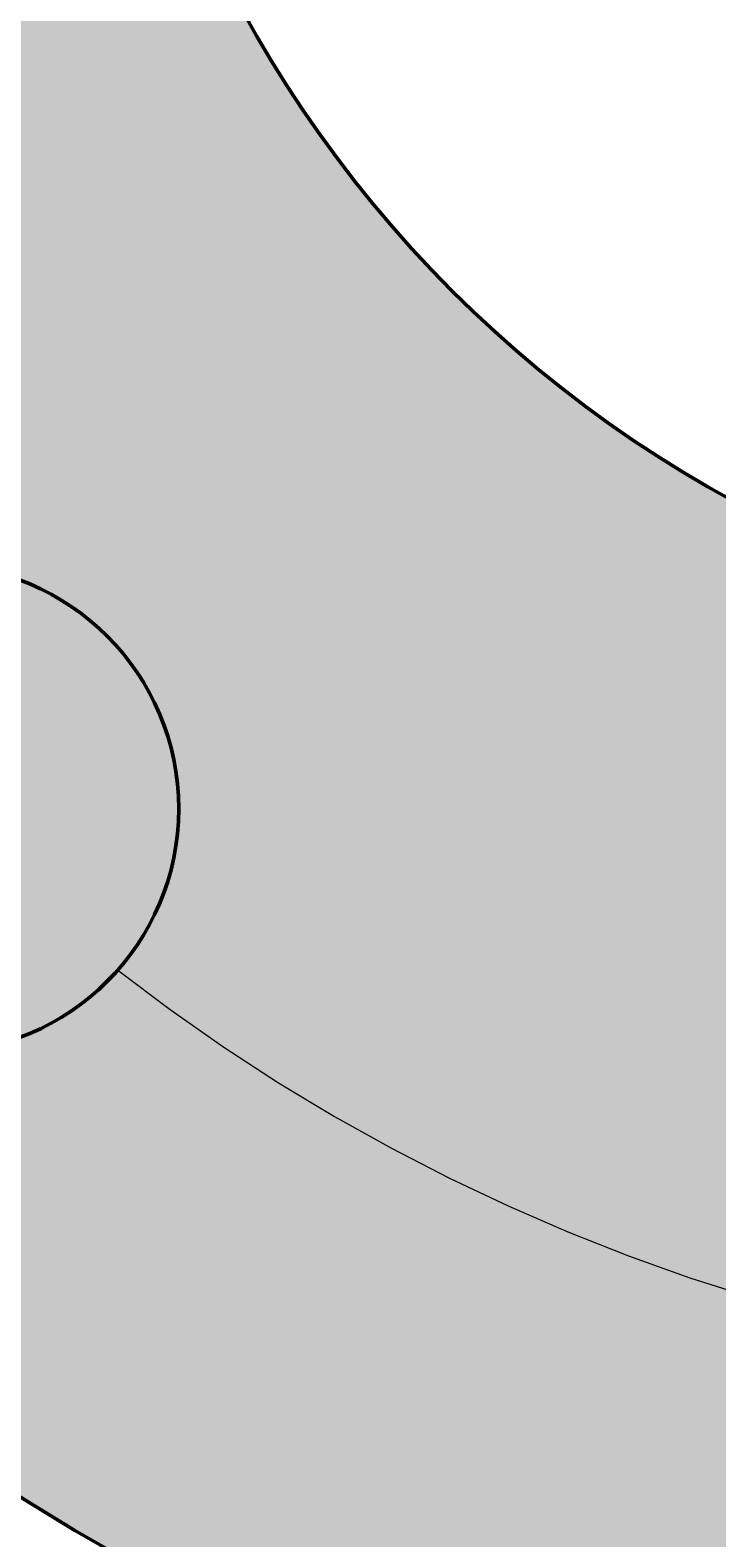
# Model space of a CAD drawing. Units: inches. Extents: x 139261 to 139415, y 52839 to 52963.
# Tile 8 of 20: x 139314 to 139328, y 52857 to 52888. Entities that reach past the tile are written whole.
import ezdxf

# ---------------------------------------------------------------- set-up
doc = ezdxf.new("R2010")
doc.units = ezdxf.units.IN
doc.header["$MEASUREMENT"] = 0
doc.linetypes.add('CENTER', pattern=[50.8, 31.75, -6.35, 6.35, -6.35])
for name, color, linetype, lineweight in [('M-CNTR', 4, 'CENTER', 18), ('M-DIMS', 2, 'Continuous', 25), ('M-HATC', 8, 'Continuous', 18), ('M-OUTL', 7, 'Continuous', 50)]:
    doc.layers.add(name, color=color, linetype=linetype, lineweight=lineweight)
doc.styles.get("Standard").update_dxf_attribs({"font": 'arial.ttf'})
doc.dimstyles.get("Standard").update_dxf_attribs({"dimtxt": 0.18, "dimasz": 0.18, "dimexe": 0.18, "dimexo": 0.0625, "dimgap": 0.09, "dimtad": 0, "dimtih": 1, "dimtoh": 1, "dimdec": 4, "dimzin": 0, "dimdsep": 46, "dimtxsty": 'Standard', "dimcen": 0.09, "dimadec": 0, "dimazin": 0, "dimtfac": 1, "dimtdec": 4, "dimtofl": 0, "dimtmove": 0, "dimatfit": 3, "dimfxl": 1, "dimtolj": 1, "dimtzin": 0, "dimarcsym": 0})

# ---------------------------------------------------------------- blocks, each defined once
blk = doc.blocks.new('*U1')
blk.add_circle((0, 0), 5)
blk = doc.blocks.new('*U2')
at = {"layer": 'M-OUTL', "color": 0, "linetype": 'ByBlock', "lineweight": -2, "transparency": 16777216, "rotation": 135}
blk.add_blockref('*U1', (139312.073, 52871.933), dxfattribs=at)
blk = doc.blocks.new('*D4')
at = {"layer": 'Defpoints', "color": 0, "transparency": 16777216}
for p in [(139373.053, 52923.26), (139307.661, 52877.175)]:
    blk.add_point(p, dxfattribs=at)
at = {"layer": 'M-DIMS', "color": 0, "lineweight": -2, "transparency": 16777216}
for p, q in [((139414.011, 52952.126), (139373.2, 52923.364)), ((139414.191, 52952.126), (139414.011, 52952.126)), ((139340.357, 52900.127), (139340.357, 52900.307)), ((139340.267, 52900.217), (139340.447, 52900.217))]:
    blk.add_line(p, q, dxfattribs=at)
blk.add_arc((139340.357, 52900.217), 40, 34.9168, 52.0771, dxfattribs=at)
at = {"layer": 'M-DIMS', "color": 0, "transparency": 16777216}
blk.add_solid([(139373.183, 52923.388), (139373.217, 52923.339), (139373.053, 52923.26)], dxfattribs=at)
at = {"layer": 'M-DIMS', "color": 0, "transparency": 16777216, "insert": (139414.822, 52952.126), "char_height": 0.18, "attachment_point": 5}
blk.add_mtext('\\A1;∅80.0000', dxfattribs=at)
blk = doc.blocks.new('*D7')
at = {"layer": 'Defpoints', "color": 0, "transparency": 16777216}
for p in [(139316.56, 52874.138), (139307.585, 52869.728)]:
    blk.add_point(p, dxfattribs=at)
at = {"layer": 'M-DIMS', "color": 0, "lineweight": -2, "transparency": 16777216}
for p, q in [((139311.983, 52871.933), (139312.163, 52871.933)), ((139312.073, 52871.843), (139312.073, 52872.023)), ((139282.904, 52857.598), (139307.424, 52869.649)), ((139282.724, 52857.598), (139282.904, 52857.598))]:
    blk.add_line(p, q, dxfattribs=at)
at = {"layer": 'M-DIMS', "color": 0, "transparency": 16777216}
blk.add_solid([(139307.41, 52869.675), (139307.437, 52869.622), (139307.585, 52869.728)], dxfattribs=at)
at = {"layer": 'M-DIMS', "color": 0, "transparency": 16777216, "insert": (139282.093, 52857.598), "char_height": 0.18, "attachment_point": 5}
blk.add_mtext('\\A1;∅10.0000', dxfattribs=at)
blk = doc.blocks.new('*D9')
at = {"layer": 'Defpoints', "color": 0, "transparency": 16777216}
for p in [(139302.054, 52932.357), (139378.659, 52868.078)]:
    blk.add_point(p, dxfattribs=at)
at = {"layer": 'M-DIMS', "color": 0, "lineweight": -2, "transparency": 16777216}
for p, q in [((139278.893, 52951.64), (139279.073, 52951.64)), ((139279.073, 52951.64), (139301.916, 52932.472)), ((139340.357, 52900.127), (139340.357, 52900.307)), ((139340.267, 52900.217), (139340.447, 52900.217))]:
    blk.add_line(p, q, dxfattribs=at)
at = {"layer": 'M-DIMS', "color": 0, "transparency": 16777216}
blk.add_solid([(139301.936, 52932.495), (139301.897, 52932.449), (139302.054, 52932.357)], dxfattribs=at)
at = {"layer": 'M-DIMS', "color": 0, "transparency": 16777216, "insert": (139278.506, 52951.64), "char_height": 0.18, "attachment_point": 5}
blk.add_mtext('\\A1;∅100', dxfattribs=at)
blk = doc.blocks.new('*D10')
at = {"layer": 'Defpoints', "color": 0, "transparency": 16777216}
for p in [(139325.07, 52937.181), (139355.644, 52863.254)]:
    blk.add_point(p, dxfattribs=at)
at = {"layer": 'M-DIMS', "color": 0, "lineweight": -2, "transparency": 16777216}
for p, q in [((139340.357, 52900.127), (139340.357, 52900.307)), ((139340.267, 52900.217), (139340.447, 52900.217)), ((139364.816, 52841.075), (139355.712, 52863.087)), ((139364.996, 52841.075), (139364.816, 52841.075))]:
    blk.add_line(p, q, dxfattribs=at)
at = {"layer": 'M-DIMS', "color": 0, "transparency": 16777216}
blk.add_solid([(139355.74, 52863.099), (139355.685, 52863.076), (139355.644, 52863.254)], dxfattribs=at)
at = {"layer": 'M-DIMS', "color": 0, "transparency": 16777216, "insert": (139365.312, 52841.075), "char_height": 0.18, "attachment_point": 5}
blk.add_mtext('\\A1;∅80', dxfattribs=at)

msp = doc.modelspace()

# ---------------------------------------------------------------- hatches: boundary and pattern name
at = {"layer": 'M-HATC'}
h = msp.add_hatch(color=256, dxfattribs=at)
h.dxf.hatch_style = 1
h.paths.add_polyline_path([(139290.35689, 52900.21749, 1), (139390.35689, 52900.21749, 1)])
h.paths.add_polyline_path([(139335.36666, 52939.90499, -0.01563646), (139335.35689, 52940.21749, -1), (139345.35689, 52940.21749, -0.01563646), (139345.34711, 52939.90499, -0.13461315), (139364.89157, 52931.80941, -0.691035), (139373.64116, 52928.50176, -0.21521822), (139371.94881, 52924.75216, -0.13461315), (139380.04439, 52905.20771, -0.43265224), (139385.35689, 52900.21749, -0.43265224), (139380.04439, 52895.22726, -0.13461315), (139371.94881, 52875.68281, -0.21521822), (139373.64116, 52871.93321, -0.691035), (139364.89157, 52868.62556, -0.13461315), (139345.34711, 52860.52999, -0.01563646), (139345.35689, 52860.21749, -1), (139335.35689, 52860.21749, -0.01563646), (139335.36666, 52860.52999, -0.13461315), (139315.82221, 52868.62556, -0.691035), (139307.07262, 52871.93321, -0.21521822), (139308.76496, 52875.68281, -0.13461315), (139300.66939, 52895.22726, -0.43265224), (139295.35689, 52900.21749, -0.43265224), (139300.66939, 52905.20771, -0.13461315), (139308.76496, 52924.75216, -0.21521822), (139307.07262, 52928.50176, -0.691035), (139315.82221, 52931.80941, -0.13461315)], flags=16)
h.paths.add_polyline_path([(139365.35689, 52900.21749, -1), (139315.35689, 52900.21749, -1)], flags=0)
h.paths.add_polyline_path([(139323.71474, 52911.30978), (139356.99903, 52911.30978, -0.3027197), (139356.99903, 52889.12519), (139323.71474, 52889.12519, -0.3027197)], flags=0)
h.paths.add_polyline_path([(139364.89157, 52931.80941, 0.13461315), (139345.34711, 52939.90499, -0.93933644), (139335.36666, 52939.90499, 0.13461315), (139315.82221, 52931.80941, -0.18270763), (139317.07262, 52928.50176, -0.64579494), (139308.76496, 52924.75216, 0.13461315), (139300.66939, 52905.20771, -0.39601219), (139305.35689, 52900.21749, -0.39601219), (139300.66939, 52895.22726, 0.13461315), (139308.76496, 52875.68281, -0.64579494), (139317.07262, 52871.93321, -0.18270763), (139315.82221, 52868.62556, 0.13461315), (139335.36666, 52860.52999, -0.93933644), (139345.34711, 52860.52999, 0.13461315), (139364.89157, 52868.62556, -0.18270763), (139363.64116, 52871.93321, -0.64579494), (139371.94881, 52875.68281, 0.13461315), (139380.04439, 52895.22726, -0.39601219), (139375.35689, 52900.21749, -0.39601219), (139380.04439, 52905.20771, 0.13461315), (139371.94881, 52924.75216, -0.64579494), (139363.64116, 52928.50176, -0.18270763)], flags=0)
h = msp.add_hatch(color=256, dxfattribs=at)
h.dxf.hatch_style = 1
h.set_gradient(color1=(205, 105, 40), tint=1)
h.paths.add_polyline_path([(139335.35689, 52940.21749, 1), (139345.35689, 52940.21749, 1)])
h.paths.add_polyline_path([(139307.07262, 52928.50176, 1), (139317.07262, 52928.50176, 1)])
h.paths.add_polyline_path([(139295.35689, 52900.21749, 1), (139305.35689, 52900.21749, 1)])
h.paths.add_polyline_path([(139307.07262, 52871.93321, 1), (139317.07262, 52871.93321, 1)])
h.paths.add_polyline_path([(139345.35689, 52860.21749, 1), (139335.35689, 52860.21749, 1)])
h.paths.add_polyline_path([(139363.64116, 52871.93321, 1), (139373.64116, 52871.93321, 1)])
h.paths.add_polyline_path([(139375.35689, 52900.21749, 1), (139385.35689, 52900.21749, 1)])
h.paths.add_polyline_path([(139363.64116, 52928.50176, 1), (139373.64116, 52928.50176, 1)])
h = msp.add_hatch(color=256, dxfattribs=at)
h.dxf.hatch_style = 1
h.paths.add_polyline_path([(139345.34711, 52939.90499, -0.93933644), (139335.36666, 52939.90499, 0.13461315), (139315.82221, 52931.80941, -0.18270763), (139317.07262, 52928.50176, -0.64579494), (139308.76496, 52924.75216, 0.13461315), (139300.66939, 52905.20771, -0.39601219), (139305.35689, 52900.21749, -0.39601219), (139300.66939, 52895.22726, 0.13461315), (139308.76496, 52875.68281, -0.64579494), (139317.07262, 52871.93321, -0.18270763), (139315.82221, 52868.62556, 0.13461315), (139335.36666, 52860.52999, -0.93933644), (139345.34711, 52860.52999, 0.13461315), (139364.89157, 52868.62556, -0.18270763), (139363.64116, 52871.93321, -0.64579494), (139371.94881, 52875.68281, 0.13461315), (139380.04439, 52895.22726, -0.39601219), (139375.35689, 52900.21749, -0.39601219), (139380.04439, 52905.20771, 0.13461315), (139371.94881, 52924.75216, -0.64579494), (139363.64116, 52928.50176, -0.18270763), (139364.89157, 52931.80941, 0.13461315)])
h.paths.add_polyline_path([(139365.35689, 52900.21749, -1), (139315.35689, 52900.21749, -1)], flags=16)
h.paths.add_polyline_path([(139356.99903, 52911.30978, -0.3027197), (139356.99903, 52889.12519), (139323.71474, 52889.12519, -0.3027197), (139323.71474, 52911.30978)], flags=0)

# ---------------------------------------------------------------- linework, layer by layer
at = {"layer": 'M-CNTR'}
msp.add_arc((139340.35689, 52900.21749), 40, 232.166643, 262.833357, dxfattribs=at)
at = {"layer": 'M-OUTL'}
for radius in [50, 25]:
    msp.add_circle((139340.35689, 52900.21749), radius, dxfattribs=at)

# ---------------------------------------------------------------- block references
msp.add_blockref('*U2', (0, 0), dxfattribs=at)

# ---------------------------------------------------------------- dimensions: what is measured, and where the dimension line sits
at = {"layer": 'M-DIMS'}
for p1, p2, override, picture, middle in [((139307.66087, 52877.17469), (139373.0529, 52923.26028), {"dimclrd": 0, "dimclre": 0, "dimclrt": 0}, '*D4', (139414.82217, 52952.12585)), ((139378.65939, 52868.07845), (139302.05438, 52932.35652), {"dimdec": 0, "dimlfac": 1, "dimrnd": 0, "dimzin": 0, "dimdsep": 46, "dimlunit": 2}, '*D9', (139278.50641, 52951.63995)), ((139325.07023, 52937.18123), (139355.64354, 52863.25374), {"dimdec": 0, "dimlfac": 1, "dimrnd": 0, "dimzin": 0, "dimdsep": 46, "dimlunit": 2}, '*D10', (139365.31206, 52841.0755)), ((139316.56001, 52874.1385), (139307.58522, 52869.72793), {"dimclrd": 0, "dimclre": 0, "dimclrt": 0}, '*D7', (139282.09259, 52857.59849))]:
    dim = msp.add_diameter_dim_2p(p1=p1, p2=p2, dimstyle='Standard', override=override, dxfattribs=at)
    dim.commit()
    dim.dimension.update_dxf_attribs({"geometry": picture, "text_midpoint": middle, "dimtype": 163})

doc.saveas('drawing.dxf')
